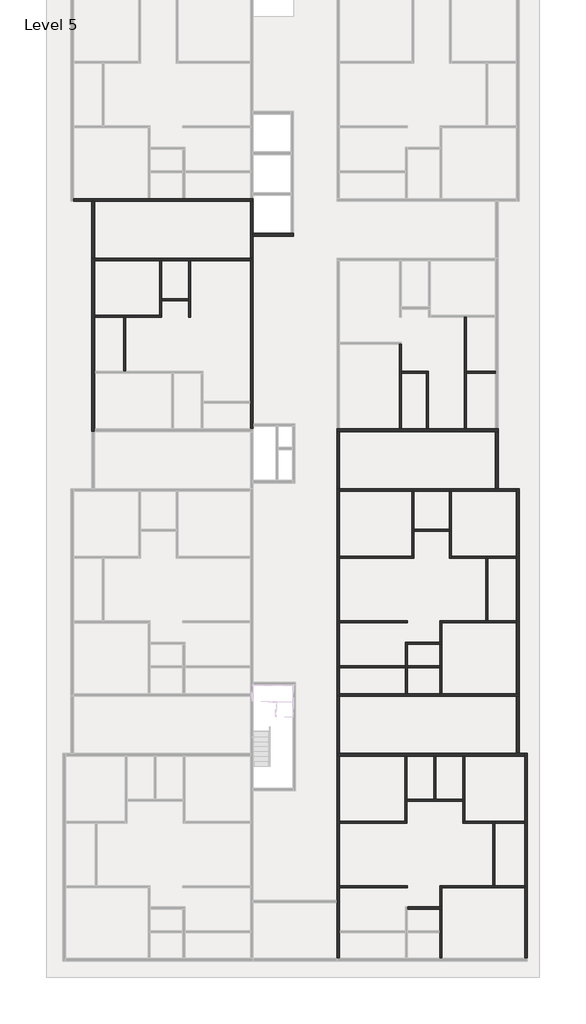
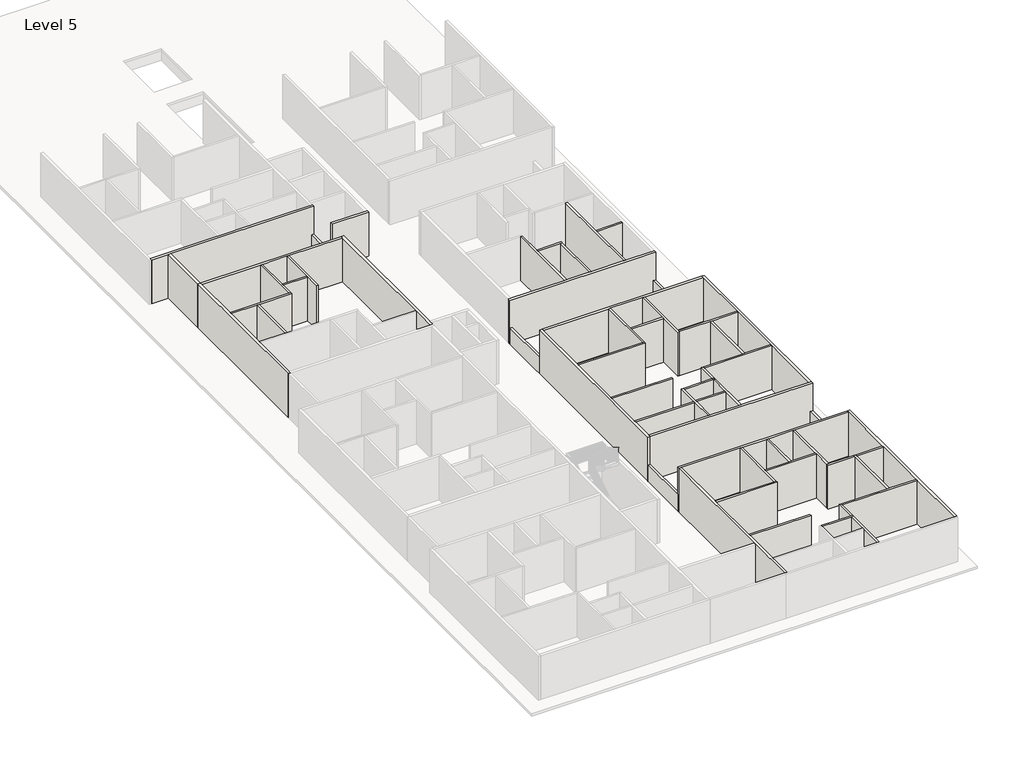
# One storey, part 2 of 8: 56 walls.
"""IFC4 building model written with IfcOpenShell, lengths in millimetres."""

from ifc_helpers import new_model, si_unit, frame, origin, place, context, project, spatial, polyline, outline, extrude, faceted_brep, element, save

model = new_model("IFC4")

# Units and contexts
model_context = context("Model", 3, world=origin())
ifc_project = project(units=[si_unit("LENGTHUNIT", "METRE", prefix="MILLI")], contexts=[model_context])

# Site, building, storey
site = spatial("IfcSite", under=ifc_project)
building = spatial("IfcBuilding", under=site)
storey = spatial("IfcBuildingStorey", under=building, Name="Level 5", Elevation=37426.6172466)

# Walls
placement = place(None, origin())
element("IfcWall", 1, ObjectType="4.5\"", at=placement, inside=storey, context=model_context, shape_type="Brep", body=[
    faceted_brep([(-12531.5544854, 2100.0216096, 37426.6172466), (-10907.2415084, 2100.0216096, 37426.6172466), (-10792.9415084, 2100.0216096, 37426.6172466), (-8759.6544854, 2100.0216096, 37426.6172466), (-8759.6544854, 2100.0216096, 40474.6172466), (-10792.9415084, 2100.0216096, 40474.6172466), (-10907.2415084, 2100.0216096, 40474.6172466), (-12531.5544854, 2100.0216096, 40474.6172466), (-12531.5544854, 2214.3216096, 37426.6172466), (-12531.5544854, 2214.3216096, 40474.6172466), (-8873.9544854, 2214.3216096, 40474.6172466), (-8759.6544854, 2214.3216096, 40474.6172466), (-8759.6544854, 2214.3216096, 37426.6172466), (-8873.9544854, 2214.3216096, 37426.6172466)], [[[0, 1, 2, 3, 4, 5, 6, 7]], [[8, 9, 10, 11, 12, 13]], [[3, 2, 1, 0, 8, 13, 12]], [[0, 7, 9, 8]], [[4, 3, 12, 11]], [[7, 6, 5, 4, 11, 10, 9]]]),
])
element("IfcWall", 2, ObjectType="4.5\"", at=placement, inside=storey, context=model_context, shape_type="Brep", body=[
    faceted_brep([(-8759.6544854, 2214.3216096, 37426.6172466), (-8759.6544854, 3014.4216096, 37426.6172466), (-8759.6544854, 3128.7216096, 37426.6172466), (-8759.6544854, 5264.2743917, 37426.6172466), (-8759.6544854, 5264.2743917, 40474.6172466), (-8759.6544854, 3128.7216096, 40474.6172466), (-8759.6544854, 3014.4216096, 40474.6172466), (-8759.6544854, 2214.3216096, 40474.6172466), (-8873.9544854, 2214.3216096, 37426.6172466), (-8873.9544854, 2214.3216096, 40474.6172466), (-8873.9544854, 5264.2743917, 40474.6172466), (-8873.9544854, 5264.2743917, 37426.6172466)], [[[0, 1, 2, 3, 4, 5, 6, 7]], [[8, 9, 10, 11]], [[3, 2, 1, 0, 8, 11]], [[0, 7, 9, 8]], [[4, 3, 11, 10]], [[7, 6, 5, 4, 10, 9]]]),
])
element("IfcWall", 3, ObjectType="4.5\"", at=placement, inside=storey, context=model_context, shape_type="Brep", body=[
    faceted_brep([(-7235.6544854, 5264.2743917, 37426.6172466), (-7235.6544854, 3128.7216096, 37426.6172466), (-7235.6544854, 3014.4216096, 37426.6172466), (-7235.6544854, 2100.0216096, 37426.6172466), (-7235.6544854, 2100.0216096, 40474.6172466), (-7235.6544854, 3014.4216096, 40474.6172466), (-7235.6544854, 3128.7216096, 40474.6172466), (-7235.6544854, 5264.2743917, 40474.6172466), (-7121.3544854, 5264.2743917, 37426.6172466), (-7121.3544854, 5264.2743917, 40474.6172466), (-7121.3544854, 2100.0216096, 40474.6172466), (-7121.3544854, 2100.0216096, 37426.6172466)], [[[0, 1, 2, 3, 4, 5, 6, 7]], [[8, 9, 10, 11]], [[3, 2, 1, 0, 8, 11]], [[4, 3, 11, 10]], [[0, 7, 9, 8]], [[7, 6, 5, 4, 10, 9]]]),
])
element("IfcWall", 4, ObjectType="4.5\"", at=placement, inside=storey, context=model_context, shape_type="SweptSolid", body=[
    extrude(outline(polyline([(-7235.6544854, 3014.4216096), (-8759.6544854, 3014.4216096), (-8759.6544854, 3128.7216096), (-7235.6544854, 3128.7216096), (-7235.6544854, 3014.4216096)])), frame((0.0, 0.0, 37426.6172466), z_axis=(0.0, 0.0, 1.0), x_axis=(1.0, 0.0, 0.0)), (0.0, 0.0, 1.0), 3048.0),
])
element("IfcWall", 5, ObjectType="4.5\"", at=placement, inside=storey, context=model_context, shape_type="SweptSolid", body=[
    extrude(outline(polyline([(-10907.2415084, -947.4344126), (-10907.2415084, 2100.0216096), (-10792.9415084, 2100.0216096), (-10792.9415084, -947.4344126), (-10907.2415084, -947.4344126)])), frame((0.0, 0.0, 37426.6172466), z_axis=(0.0, 0.0, 1.0), x_axis=(1.0, 0.0, 0.0)), (0.0, 0.0, 1.0), 3048.0),
])
element("IfcWall", 6, ObjectType="4.5\"", at=placement, inside=storey, context=model_context, shape_type="Brep", body=[
    faceted_brep([(5056.6584916, -31173.4344126, 37426.6172466), (6885.4584916, -31173.4344126, 37426.6172466), (6999.7584916, -31173.4344126, 37426.6172466), (6999.7584916, -31173.4344126, 40474.6172466), (6885.4584916, -31173.4344126, 40474.6172466), (5056.6584916, -31173.4344126, 40474.6172466), (5056.6584916, -31059.1344126, 37426.6172466), (5056.6584916, -31059.1344126, 40474.6172466), (6885.4584916, -31059.1344126, 40474.6172466), (6999.7584916, -31059.1344126, 40474.6172466), (6999.7584916, -31059.1344126, 37426.6172466), (6885.4584916, -31059.1344126, 37426.6172466)], [[[0, 1, 2, 3, 4, 5]], [[6, 7, 8, 9, 10, 11]], [[2, 1, 0, 6, 11, 10]], [[0, 5, 7, 6]], [[3, 2, 10, 9]], [[5, 4, 3, 9, 8, 7]]]),
])
element("IfcWall", 7, ObjectType="4.5\"", at=placement, inside=storey, context=model_context, shape_type="Brep", body=[
    faceted_brep([(6885.4584916, -31173.4344126, 37426.6172466), (6885.4584916, -32392.6344126, 37426.6172466), (6885.4584916, -32506.9344126, 37426.6172466), (6885.4584916, -33954.7344126, 37426.6172466), (6885.4584916, -33954.7344126, 40474.6172466), (6885.4584916, -32506.9344126, 40474.6172466), (6885.4584916, -32392.6344126, 40474.6172466), (6885.4584916, -31173.4344126, 40474.6172466), (6999.7584916, -31173.4344126, 37426.6172466), (6999.7584916, -31173.4344126, 40474.6172466), (6999.7584916, -33954.7344126, 40474.6172466), (6999.7584916, -33954.7344126, 37426.6172466)], [[[0, 1, 2, 3, 4, 5, 6, 7]], [[8, 9, 10, 11]], [[3, 2, 1, 0, 8, 11]], [[0, 7, 9, 8]], [[4, 3, 11, 10]], [[7, 6, 5, 4, 10, 9]]]),
])
element("IfcWall", 8, ObjectType="4.5\"", at=placement, inside=storey, context=model_context, shape_type="Brep", body=[
    faceted_brep([(6999.7584916, -31059.1344126, 37426.6172466), (6999.7584916, -29966.9344126, 37426.6172466), (6999.7584916, -29852.6344126, 37426.6172466), (6999.7584916, -29852.6344126, 40474.6172466), (6999.7584916, -29966.9344126, 40474.6172466), (6999.7584916, -31059.1344126, 40474.6172466), (6885.4584916, -31059.1344126, 37426.6172466), (6885.4584916, -31059.1344126, 40474.6172466), (6885.4584916, -29852.6344126, 40474.6172466), (6885.4584916, -29852.6344126, 37426.6172466)], [[[0, 1, 2, 3, 4, 5]], [[6, 7, 8, 9]], [[2, 1, 0, 6, 9]], [[0, 5, 7, 6]], [[3, 2, 9, 8]], [[5, 4, 3, 8, 7]]]),
])
element("IfcWall", 9, ObjectType="4.5\"", at=placement, inside=storey, context=model_context, shape_type="Brep", body=[
    faceted_brep([(6999.7584916, -29966.9344126, 37426.6172466), (11660.6584916, -29966.9344126, 37426.6172466), (11660.6584916, -29966.9344126, 40474.6172466), (6999.7584916, -29966.9344126, 40474.6172466), (6999.7584916, -29852.6344126, 37426.6172466), (6999.7584916, -29852.6344126, 40474.6172466), (9869.9584916, -29852.6344126, 40474.6172466), (9984.2584916, -29852.6344126, 40474.6172466), (11660.6584916, -29852.6344126, 40474.6172466), (11660.6584916, -29852.6344126, 37426.6172466), (9984.2584916, -29852.6344126, 37426.6172466), (9869.9584916, -29852.6344126, 37426.6172466)], [[[0, 1, 2, 3]], [[4, 5, 6, 7, 8, 9, 10, 11]], [[1, 0, 4, 11, 10, 9]], [[0, 3, 5, 4]], [[2, 1, 9, 8]], [[3, 2, 8, 7, 6, 5]]]),
])
element("IfcWall", 10, ObjectType="4.5\"", at=placement, inside=storey, context=model_context, shape_type="SweptSolid", body=[
    extrude(outline(polyline([(5056.6584916, -29966.9344126), (1259.3584916, -29966.9344126), (1259.3584916, -29852.6344126), (5056.6584916, -29852.6344126), (5056.6584916, -29966.9344126)])), frame((0.0, 0.0, 37426.6172466), z_axis=(0.0, 0.0, 1.0), x_axis=(1.0, 0.0, 0.0)), (0.0, 0.0, 1.0), 3048.0),
])
element("IfcWall", 11, ObjectType="4.5\"", at=placement, inside=storey, context=model_context, shape_type="Brep", body=[
    faceted_brep([(1259.3584916, -26347.4344126, 37426.6172466), (5031.2584916, -26347.4344126, 37426.6172466), (5031.2584916, -26347.4344126, 40474.6172466), (1259.3584916, -26347.4344126, 40474.6172466), (1259.3584916, -26233.1344126, 37426.6172466), (1259.3584916, -26233.1344126, 40474.6172466), (4916.9584916, -26233.1344126, 40474.6172466), (5031.2584916, -26233.1344126, 40474.6172466), (5031.2584916, -26233.1344126, 37426.6172466), (4916.9584916, -26233.1344126, 37426.6172466)], [[[0, 1, 2, 3]], [[4, 5, 6, 7, 8, 9]], [[1, 0, 4, 9, 8]], [[0, 3, 5, 4]], [[2, 1, 8, 7]], [[3, 2, 7, 6, 5]]]),
])
element("IfcWall", 12, ObjectType="4.5\"", at=placement, inside=storey, context=model_context, shape_type="Brep", body=[
    faceted_brep([(5031.2584916, -26233.1344126, 37426.6172466), (5031.2584916, -25128.2344126, 37426.6172466), (5031.2584916, -25013.9344126, 37426.6172466), (5031.2584916, -22575.5344126, 37426.6172466), (5031.2584916, -22575.5344126, 40474.6172466), (5031.2584916, -25013.9344126, 40474.6172466), (5031.2584916, -25128.2344126, 40474.6172466), (5031.2584916, -26233.1344126, 40474.6172466), (4916.9584916, -26233.1344126, 37426.6172466), (4916.9584916, -26233.1344126, 40474.6172466), (4916.9584916, -22575.5344126, 40474.6172466), (4916.9584916, -22575.5344126, 37426.6172466)], [[[0, 1, 2, 3, 4, 5, 6, 7]], [[8, 9, 10, 11]], [[3, 2, 1, 0, 8, 11]], [[0, 7, 9, 8]], [[4, 3, 11, 10]], [[7, 6, 5, 4, 10, 9]]]),
])
element("IfcWall", 13, ObjectType="4.5\"", at=placement, inside=storey, context=model_context, shape_type="Brep", body=[
    faceted_brep([(9984.2584916, -29852.6344126, 37426.6172466), (9984.2584916, -26347.4344126, 37426.6172466), (9984.2584916, -26233.1344126, 37426.6172466), (9984.2584916, -26233.1344126, 40474.6172466), (9984.2584916, -26347.4344126, 40474.6172466), (9984.2584916, -29852.6344126, 40474.6172466), (9869.9584916, -29852.6344126, 37426.6172466), (9869.9584916, -29852.6344126, 40474.6172466), (9869.9584916, -26347.4344126, 40474.6172466), (9869.9584916, -26233.1344126, 40474.6172466), (9869.9584916, -26233.1344126, 37426.6172466), (9869.9584916, -26347.4344126, 37426.6172466)], [[[0, 1, 2, 3, 4, 5]], [[6, 7, 8, 9, 10, 11]], [[2, 1, 0, 6, 11, 10]], [[0, 5, 7, 6]], [[3, 2, 10, 9]], [[5, 4, 3, 9, 8, 7]]]),
])
element("IfcWall", 14, ObjectType="4.5\"", at=placement, inside=storey, context=model_context, shape_type="SweptSolid", body=[
    extrude(outline(polyline([(11660.6584916, -26347.4344126), (9984.2584916, -26347.4344126), (9984.2584916, -26233.1344126), (11660.6584916, -26233.1344126), (11660.6584916, -26347.4344126)])), frame((0.0, 0.0, 37426.6172466), z_axis=(0.0, 0.0, 1.0), x_axis=(1.0, 0.0, 0.0)), (0.0, 0.0, 1.0), 3048.0),
])
element("IfcWall", 15, ObjectType="4.5\"", at=placement, inside=storey, context=model_context, shape_type="Brep", body=[
    faceted_brep([(9869.9584916, -26233.1344126, 37426.6172466), (8307.8584916, -26233.1344126, 37426.6172466), (8193.5584916, -26233.1344126, 37426.6172466), (8193.5584916, -26233.1344126, 40474.6172466), (8307.8584916, -26233.1344126, 40474.6172466), (9869.9584916, -26233.1344126, 40474.6172466), (9869.9584916, -26347.4344126, 37426.6172466), (9869.9584916, -26347.4344126, 40474.6172466), (8193.5584916, -26347.4344126, 40474.6172466), (8193.5584916, -26347.4344126, 37426.6172466)], [[[0, 1, 2, 3, 4, 5]], [[6, 7, 8, 9]], [[2, 1, 0, 6, 9]], [[0, 5, 7, 6]], [[3, 2, 9, 8]], [[5, 4, 3, 8, 7]]]),
])
element("IfcWall", 16, ObjectType="4.5\"", at=placement, inside=storey, context=model_context, shape_type="Brep", body=[
    faceted_brep([(8307.8584916, -26233.1344126, 37426.6172466), (8307.8584916, -22575.5344126, 37426.6172466), (8307.8584916, -22575.5344126, 40474.6172466), (8307.8584916, -26233.1344126, 40474.6172466), (8193.5584916, -26233.1344126, 37426.6172466), (8193.5584916, -26233.1344126, 40474.6172466), (8193.5584916, -25128.2344126, 40474.6172466), (8193.5584916, -25013.9344126, 40474.6172466), (8193.5584916, -22575.5344126, 40474.6172466), (8193.5584916, -22575.5344126, 37426.6172466), (8193.5584916, -25013.9344126, 37426.6172466), (8193.5584916, -25128.2344126, 37426.6172466)], [[[0, 1, 2, 3]], [[4, 5, 6, 7, 8, 9, 10, 11]], [[1, 0, 4, 11, 10, 9]], [[0, 3, 5, 4]], [[2, 1, 9, 8]], [[3, 2, 8, 7, 6, 5]]]),
])
element("IfcWall", 17, ObjectType="4.5\"", at=placement, inside=storey, context=model_context, shape_type="Brep", body=[
    faceted_brep([(5031.2584916, -25128.2344126, 37426.6172466), (8193.5584916, -25128.2344126, 37426.6172466), (8193.5584916, -25128.2344126, 40474.6172466), (5031.2584916, -25128.2344126, 40474.6172466), (5031.2584916, -25013.9344126, 37426.6172466), (5031.2584916, -25013.9344126, 40474.6172466), (6555.2584916, -25013.9344126, 40474.6172466), (6669.5584916, -25013.9344126, 40474.6172466), (8193.5584916, -25013.9344126, 40474.6172466), (8193.5584916, -25013.9344126, 37426.6172466), (6669.5584916, -25013.9344126, 37426.6172466), (6555.2584916, -25013.9344126, 37426.6172466)], [[[0, 1, 2, 3]], [[4, 5, 6, 7, 8, 9, 10, 11]], [[1, 0, 4, 11, 10, 9]], [[0, 3, 5, 4]], [[2, 1, 9, 8]], [[3, 2, 8, 7, 6, 5]]]),
])
element("IfcWall", 18, ObjectType="4.5\"", at=placement, inside=storey, context=model_context, shape_type="SweptSolid", body=[
    extrude(outline(polyline([(6555.2584916, -25013.9344126), (6555.2584916, -22575.5344126), (6669.5584916, -22575.5344126), (6669.5584916, -25013.9344126), (6555.2584916, -25013.9344126)])), frame((0.0, 0.0, 37426.6172466), z_axis=(0.0, 0.0, 1.0), x_axis=(1.0, 0.0, 0.0)), (0.0, 0.0, 1.0), 3048.0),
])
element("IfcWall", 19, ObjectType="4.5\"", at=placement, inside=storey, context=model_context, shape_type="SweptSolid", body=[
    extrude(outline(polyline([(4942.3584916, -17622.5344126), (1259.3584916, -17622.5344126), (1259.3584916, -17508.2344126), (4942.3584916, -17508.2344126), (4942.3584916, -17622.5344126)])), frame((0.0, 0.0, 37426.6172466), z_axis=(0.0, 0.0, 1.0), x_axis=(1.0, 0.0, 0.0)), (0.0, 0.0, 1.0), 3048.0),
])
element("IfcWall", 20, ObjectType="4.5\"", at=placement, inside=storey, context=model_context, shape_type="Brep", body=[
    faceted_brep([(4942.3584916, -16174.7344126, 37426.6172466), (4942.3584916, -17508.2344126, 37426.6172466), (4942.3584916, -17622.5344126, 37426.6172466), (4942.3584916, -19070.3344126, 37426.6172466), (4942.3584916, -19070.3344126, 40474.6172466), (4942.3584916, -17622.5344126, 40474.6172466), (4942.3584916, -17508.2344126, 40474.6172466), (4942.3584916, -16174.7344126, 40474.6172466), (5056.6584916, -16174.7344126, 37426.6172466), (5056.6584916, -16174.7344126, 40474.6172466), (5056.6584916, -16289.0344126, 40474.6172466), (5056.6584916, -17508.2344126, 40474.6172466), (5056.6584916, -17622.5344126, 40474.6172466), (5056.6584916, -19070.3344126, 40474.6172466), (5056.6584916, -19070.3344126, 37426.6172466), (5056.6584916, -17622.5344126, 37426.6172466), (5056.6584916, -17508.2344126, 37426.6172466), (5056.6584916, -16289.0344126, 37426.6172466)], [[[0, 1, 2, 3, 4, 5, 6, 7]], [[8, 9, 10, 11, 12, 13, 14, 15, 16, 17]], [[3, 2, 1, 0, 8, 17, 16, 15, 14]], [[4, 3, 14, 13]], [[0, 7, 9, 8]], [[7, 6, 5, 4, 13, 12, 11, 10, 9]]]),
])
element("IfcWall", 21, ObjectType="4.5\"", at=placement, inside=storey, context=model_context, shape_type="Brep", body=[
    faceted_brep([(5056.6584916, -16289.0344126, 37426.6172466), (6885.4584916, -16289.0344126, 37426.6172466), (6999.7584916, -16289.0344126, 37426.6172466), (6999.7584916, -16289.0344126, 40474.6172466), (6885.4584916, -16289.0344126, 40474.6172466), (5056.6584916, -16289.0344126, 40474.6172466), (5056.6584916, -16174.7344126, 37426.6172466), (5056.6584916, -16174.7344126, 40474.6172466), (6885.4584916, -16174.7344126, 40474.6172466), (6999.7584916, -16174.7344126, 40474.6172466), (6999.7584916, -16174.7344126, 37426.6172466), (6885.4584916, -16174.7344126, 37426.6172466)], [[[0, 1, 2, 3, 4, 5]], [[6, 7, 8, 9, 10, 11]], [[2, 1, 0, 6, 11, 10]], [[0, 5, 7, 6]], [[3, 2, 10, 9]], [[5, 4, 3, 9, 8, 7]]]),
])
element("IfcWall", 22, ObjectType="4.5\"", at=placement, inside=storey, context=model_context, shape_type="Brep", body=[
    faceted_brep([(6885.4584916, -16289.0344126, 37426.6172466), (6885.4584916, -17508.2344126, 37426.6172466), (6885.4584916, -17622.5344126, 37426.6172466), (6885.4584916, -19070.3344126, 37426.6172466), (6885.4584916, -19070.3344126, 40474.6172466), (6885.4584916, -17622.5344126, 40474.6172466), (6885.4584916, -17508.2344126, 40474.6172466), (6885.4584916, -16289.0344126, 40474.6172466), (6999.7584916, -16289.0344126, 37426.6172466), (6999.7584916, -16289.0344126, 40474.6172466), (6999.7584916, -19070.3344126, 40474.6172466), (6999.7584916, -19070.3344126, 37426.6172466)], [[[0, 1, 2, 3, 4, 5, 6, 7]], [[8, 9, 10, 11]], [[3, 2, 1, 0, 8, 11]], [[0, 7, 9, 8]], [[4, 3, 11, 10]], [[7, 6, 5, 4, 10, 9]]]),
])
element("IfcWall", 23, ObjectType="4.5\"", at=placement, inside=storey, context=model_context, shape_type="SweptSolid", body=[
    extrude(outline(polyline([(6885.4584916, -17622.5344126), (5056.6584916, -17622.5344126), (5056.6584916, -17508.2344126), (6885.4584916, -17508.2344126), (6885.4584916, -17622.5344126)])), frame((0.0, 0.0, 37426.6172466), z_axis=(0.0, 0.0, 1.0), x_axis=(1.0, 0.0, 0.0)), (0.0, 0.0, 1.0), 3048.0),
])
element("IfcWall", 24, ObjectType="4.5\"", at=placement, inside=storey, context=model_context, shape_type="Brep", body=[
    faceted_brep([(6999.7584916, -16174.7344126, 37426.6172466), (6999.7584916, -15082.5344126, 37426.6172466), (6999.7584916, -14968.2344126, 37426.6172466), (6999.7584916, -14968.2344126, 40474.6172466), (6999.7584916, -15082.5344126, 40474.6172466), (6999.7584916, -16174.7344126, 40474.6172466), (6885.4584916, -16174.7344126, 37426.6172466), (6885.4584916, -16174.7344126, 40474.6172466), (6885.4584916, -14968.2344126, 40474.6172466), (6885.4584916, -14968.2344126, 37426.6172466)], [[[0, 1, 2, 3, 4, 5]], [[6, 7, 8, 9]], [[2, 1, 0, 6, 9]], [[0, 5, 7, 6]], [[3, 2, 9, 8]], [[5, 4, 3, 8, 7]]]),
])
element("IfcWall", 25, ObjectType="4.5\"", at=placement, inside=storey, context=model_context, shape_type="Brep", body=[
    faceted_brep([(6999.7584916, -15082.5344126, 37426.6172466), (11208.5214687, -15082.5344126, 37426.6172466), (11208.5214687, -15082.5344126, 40474.6172466), (6999.7584916, -15082.5344126, 40474.6172466), (6999.7584916, -14968.2344126, 37426.6172466), (6999.7584916, -14968.2344126, 40474.6172466), (9469.9084916, -14968.2344126, 40474.6172466), (9584.2084916, -14968.2344126, 40474.6172466), (11208.5214687, -14968.2344126, 40474.6172466), (11208.5214687, -14968.2344126, 37426.6172466), (9584.2084916, -14968.2344126, 37426.6172466), (9469.9084916, -14968.2344126, 37426.6172466)], [[[0, 1, 2, 3]], [[4, 5, 6, 7, 8, 9, 10, 11]], [[1, 0, 4, 11, 10, 9]], [[0, 3, 5, 4]], [[2, 1, 9, 8]], [[3, 2, 8, 7, 6, 5]]]),
])
element("IfcWall", 26, ObjectType="4.5\"", at=placement, inside=storey, context=model_context, shape_type="SweptSolid", body=[
    extrude(outline(polyline([(5056.6584916, -15082.5344126), (1259.3584916, -15082.5344126), (1259.3584916, -14968.2344126), (5056.6584916, -14968.2344126), (5056.6584916, -15082.5344126)])), frame((0.0, 0.0, 37426.6172466), z_axis=(0.0, 0.0, 1.0), x_axis=(1.0, 0.0, 0.0)), (0.0, 0.0, 1.0), 3048.0),
])
element("IfcWall", 27, ObjectType="4.5\"", at=placement, inside=storey, context=model_context, shape_type="Brep", body=[
    faceted_brep([(1259.3584916, -11463.0344126, 37426.6172466), (5430.0214687, -11463.0344126, 37426.6172466), (5430.0214687, -11463.0344126, 40474.6172466), (1259.3584916, -11463.0344126, 40474.6172466), (1259.3584916, -11348.7344126, 37426.6172466), (1259.3584916, -11348.7344126, 40474.6172466), (5315.7214687, -11348.7344126, 40474.6172466), (5430.0214687, -11348.7344126, 40474.6172466), (5430.0214687, -11348.7344126, 37426.6172466), (5315.7214687, -11348.7344126, 37426.6172466)], [[[0, 1, 2, 3]], [[4, 5, 6, 7, 8, 9]], [[1, 0, 4, 9, 8]], [[0, 3, 5, 4]], [[2, 1, 8, 7]], [[3, 2, 7, 6, 5]]]),
])
element("IfcWall", 28, ObjectType="4.5\"", at=placement, inside=storey, context=model_context, shape_type="Brep", body=[
    faceted_brep([(5430.0214687, -11348.7344126, 37426.6172466), (5430.0214687, -9939.0344126, 37426.6172466), (5430.0214687, -9824.7344126, 37426.6172466), (5430.0214687, -7691.1344126, 37426.6172466), (5430.0214687, -7691.1344126, 40474.6172466), (5430.0214687, -9824.7344126, 40474.6172466), (5430.0214687, -9939.0344126, 40474.6172466), (5430.0214687, -11348.7344126, 40474.6172466), (5315.7214687, -11348.7344126, 37426.6172466), (5315.7214687, -11348.7344126, 40474.6172466), (5315.7214687, -7691.1344126, 40474.6172466), (5315.7214687, -7691.1344126, 37426.6172466)], [[[0, 1, 2, 3, 4, 5, 6, 7]], [[8, 9, 10, 11]], [[3, 2, 1, 0, 8, 11]], [[0, 7, 9, 8]], [[4, 3, 11, 10]], [[7, 6, 5, 4, 10, 9]]]),
])
element("IfcWall", 29, ObjectType="4.5\"", at=placement, inside=storey, context=model_context, shape_type="SweptSolid", body=[
    extrude(outline(polyline([(7436.6214687, -9939.0344126), (5430.0214687, -9939.0344126), (5430.0214687, -9824.7344126), (7436.6214687, -9824.7344126), (7436.6214687, -9939.0344126)])), frame((0.0, 0.0, 37426.6172466), z_axis=(0.0, 0.0, 1.0), x_axis=(1.0, 0.0, 0.0)), (0.0, 0.0, 1.0), 3048.0),
])
element("IfcWall", 30, ObjectType="4.5\"", at=placement, inside=storey, context=model_context, shape_type="Brep", body=[
    faceted_brep([(7436.6214687, -7691.1344126, 37426.6172466), (7436.6214687, -9824.7344126, 37426.6172466), (7436.6214687, -9939.0344126, 37426.6172466), (7436.6214687, -11463.0344126, 37426.6172466), (7436.6214687, -11463.0344126, 40474.6172466), (7436.6214687, -9939.0344126, 40474.6172466), (7436.6214687, -9824.7344126, 40474.6172466), (7436.6214687, -7691.1344126, 40474.6172466), (7550.9214687, -7691.1344126, 37426.6172466), (7550.9214687, -7691.1344126, 40474.6172466), (7550.9214687, -11348.7344126, 40474.6172466), (7550.9214687, -11463.0344126, 40474.6172466), (7550.9214687, -11463.0344126, 37426.6172466), (7550.9214687, -11348.7344126, 37426.6172466)], [[[0, 1, 2, 3, 4, 5, 6, 7]], [[8, 9, 10, 11, 12, 13]], [[3, 2, 1, 0, 8, 13, 12]], [[0, 7, 9, 8]], [[4, 3, 12, 11]], [[7, 6, 5, 4, 11, 10, 9]]]),
])
element("IfcWall", 31, ObjectType="4.5\"", at=placement, inside=storey, context=model_context, shape_type="Brep", body=[
    faceted_brep([(7550.9214687, -11463.0344126, 37426.6172466), (9469.9084916, -11463.0344126, 37426.6172466), (9584.2084916, -11463.0344126, 37426.6172466), (11208.5214687, -11463.0344126, 37426.6172466), (11208.5214687, -11463.0344126, 40474.6172466), (9584.2084916, -11463.0344126, 40474.6172466), (9469.9084916, -11463.0344126, 40474.6172466), (7550.9214687, -11463.0344126, 40474.6172466), (7550.9214687, -11348.7344126, 37426.6172466), (7550.9214687, -11348.7344126, 40474.6172466), (11208.5214687, -11348.7344126, 40474.6172466), (11208.5214687, -11348.7344126, 37426.6172466)], [[[0, 1, 2, 3, 4, 5, 6, 7]], [[8, 9, 10, 11]], [[3, 2, 1, 0, 8, 11]], [[0, 7, 9, 8]], [[4, 3, 11, 10]], [[7, 6, 5, 4, 10, 9]]]),
])
element("IfcWall", 32, ObjectType="4.5\"", at=placement, inside=storey, context=model_context, shape_type="SweptSolid", body=[
    extrude(outline(polyline([(9469.9084916, -14968.2344126), (9469.9084916, -11463.0344126), (9584.2084916, -11463.0344126), (9584.2084916, -14968.2344126), (9469.9084916, -14968.2344126)])), frame((0.0, 0.0, 37426.6172466), z_axis=(0.0, 0.0, 1.0), x_axis=(1.0, 0.0, 0.0)), (0.0, 0.0, 1.0), 3048.0),
])
element("IfcWall", 33, ObjectType="4.5\"", at=placement, inside=storey, context=model_context, shape_type="Brep", body=[
    faceted_brep([(4610.8714687, 572.7745083, 37426.6172466), (4610.8714687, -4185.9344126, 37426.6172466), (4610.8714687, -4185.9344126, 40474.6172466), (4610.8714687, 572.7745083, 40474.6172466), (4725.1714687, 572.7745083, 37426.6172466), (4725.1714687, 572.7745083, 40474.6172466), (4725.1714687, -947.4344126, 40474.6172466), (4725.1714687, -1061.7344126, 40474.6172466), (4725.1714687, -4185.9344126, 40474.6172466), (4725.1714687, -4185.9344126, 37426.6172466), (4725.1714687, -1061.7344126, 37426.6172466), (4725.1714687, -947.4344126, 37426.6172466)], [[[0, 1, 2, 3]], [[4, 5, 6, 7, 8, 9, 10, 11]], [[1, 0, 4, 11, 10, 9]], [[0, 3, 5, 4]], [[2, 1, 9, 8]], [[3, 2, 8, 7, 6, 5]]]),
])
element("IfcWall", 34, ObjectType="4.5\"", at=placement, inside=storey, context=model_context, shape_type="Brep", body=[
    faceted_brep([(4725.1714687, -1061.7344126, 37426.6172466), (6134.8714687, -1061.7344126, 37426.6172466), (6249.1714687, -1061.7344126, 37426.6172466), (6249.1714687, -1061.7344126, 40474.6172466), (6134.8714687, -1061.7344126, 40474.6172466), (4725.1714687, -1061.7344126, 40474.6172466), (4725.1714687, -947.4344126, 37426.6172466), (4725.1714687, -947.4344126, 40474.6172466), (6249.1714687, -947.4344126, 40474.6172466), (6249.1714687, -947.4344126, 37426.6172466)], [[[0, 1, 2, 3, 4, 5]], [[6, 7, 8, 9]], [[2, 1, 0, 6, 9]], [[0, 5, 7, 6]], [[3, 2, 9, 8]], [[5, 4, 3, 8, 7]]]),
])
element("IfcWall", 35, ObjectType="4.5\"", at=placement, inside=storey, context=model_context, shape_type="SweptSolid", body=[
    extrude(outline(polyline([(6134.8714687, -4185.9344126), (6134.8714687, -1061.7344126), (6249.1714687, -1061.7344126), (6249.1714687, -4185.9344126), (6134.8714687, -4185.9344126)])), frame((0.0, 0.0, 37426.6172466), z_axis=(0.0, 0.0, 1.0), x_axis=(1.0, 0.0, 0.0)), (0.0, 0.0, 1.0), 3048.0),
])
element("IfcWall", 36, ObjectType="4.5\"", at=placement, inside=storey, context=model_context, shape_type="Brep", body=[
    faceted_brep([(8396.7584916, -4185.9344126, 37426.6172466), (8396.7584916, -1061.7344126, 37426.6172466), (8396.7584916, -947.4344126, 37426.6172466), (8396.7584916, 2100.0216096, 37426.6172466), (8396.7584916, 2100.0216096, 40474.6172466), (8396.7584916, -947.4344126, 40474.6172466), (8396.7584916, -1061.7344126, 40474.6172466), (8396.7584916, -4185.9344126, 40474.6172466), (8282.4584916, -4185.9344126, 37426.6172466), (8282.4584916, -4185.9344126, 40474.6172466), (8282.4584916, 2100.0216096, 40474.6172466), (8282.4584916, 2100.0216096, 37426.6172466)], [[[0, 1, 2, 3, 4, 5, 6, 7]], [[8, 9, 10, 11]], [[3, 2, 1, 0, 8, 11]], [[0, 7, 9, 8]], [[4, 3, 11, 10]], [[7, 6, 5, 4, 10, 9]]]),
])
element("IfcWall", 37, ObjectType="4.5\"", at=placement, inside=storey, context=model_context, shape_type="SweptSolid", body=[
    extrude(outline(polyline([(8396.7584916, -947.4344126), (10021.0714687, -947.4344126), (10021.0714687, -1061.7344126), (8396.7584916, -1061.7344126), (8396.7584916, -947.4344126)])), frame((0.0, 0.0, 37426.6172466), z_axis=(0.0, 0.0, 1.0), x_axis=(1.0, 0.0, 0.0)), (0.0, 0.0, 1.0), 3048.0),
])
element("IfcWall", 38, ObjectType="6\"", at=placement, inside=storey, context=model_context, shape_type="Brep", body=[
    faceted_brep([(-13719.0044854, 8615.1216096, 37426.6172466), (-12683.9544854, 8615.1216096, 37426.6172466), (-12531.5544854, 8615.1216096, 37426.6172466), (-3769.8415084, 8615.1216096, 37426.6172466), (-3617.4415084, 8615.1216096, 37426.6172466), (-3617.4415084, 8615.1216096, 38645.8172466), (-3617.4415084, 8615.1216096, 40474.6172466), (-12531.5544854, 8615.1216096, 40474.6172466), (-12683.9544854, 8615.1216096, 40474.6172466), (-13719.0044854, 8615.1216096, 40474.6172466), (-13719.0044854, 8767.5216096, 37426.6172466), (-13719.0044854, 8767.5216096, 40474.6172466), (-9510.2415084, 8767.5216096, 40474.6172466), (-9395.9415084, 8767.5216096, 40474.6172466), (-7567.1415084, 8767.5216096, 40474.6172466), (-7452.8415084, 8767.5216096, 40474.6172466), (-3769.8415084, 8767.5216096, 40474.6172466), (-3617.4415084, 8767.5216096, 40474.6172466), (-3617.4415084, 8767.5216096, 37426.6172466), (-3769.8415084, 8767.5216096, 37426.6172466), (-7452.8415084, 8767.5216096, 37426.6172466), (-7567.1415084, 8767.5216096, 37426.6172466), (-9395.9415084, 8767.5216096, 37426.6172466), (-9510.2415084, 8767.5216096, 37426.6172466)], [[[0, 1, 2, 3, 4, 5, 6, 7, 8, 9]], [[10, 11, 12, 13, 14, 15, 16, 17, 18, 19, 20, 21, 22, 23]], [[4, 3, 2, 1, 0, 10, 23, 22, 21, 20, 19, 18]], [[0, 9, 11, 10]], [[4, 18, 17, 6, 5]], [[9, 8, 7, 6, 17, 16, 15, 14, 13, 12, 11]]]),
])
element("IfcWall", 39, ObjectType="6\"", at=placement, inside=storey, context=model_context, shape_type="Brep", body=[
    faceted_brep([(-12683.9544854, 5416.6743917, 37426.6172466), (-12683.9544854, -4338.3344126, 37426.6172466), (-12683.9544854, -4338.3344126, 40474.6172466), (-12683.9544854, 5416.6743917, 40474.6172466), (-12531.5544854, 5416.6743917, 37426.6172466), (-12531.5544854, 5416.6743917, 40474.6172466), (-12531.5544854, 5264.2743917, 40474.6172466), (-12531.5544854, 2214.3216096, 40474.6172466), (-12531.5544854, 2100.0216096, 40474.6172466), (-12531.5544854, -947.4344126, 40474.6172466), (-12531.5544854, -1061.7344126, 40474.6172466), (-12531.5544854, -4185.9344126, 40474.6172466), (-12531.5544854, -4338.3344126, 40474.6172466), (-12531.5544854, -4338.3344126, 37426.6172466), (-12531.5544854, -4185.9344126, 37426.6172466), (-12531.5544854, -1061.7344126, 37426.6172466), (-12531.5544854, -947.4344126, 37426.6172466), (-12531.5544854, 2100.0216096, 37426.6172466), (-12531.5544854, 2214.3216096, 37426.6172466), (-12531.5544854, 5264.2743917, 37426.6172466)], [[[0, 1, 2, 3]], [[4, 5, 6, 7, 8, 9, 10, 11, 12, 13, 14, 15, 16, 17, 18, 19]], [[1, 0, 4, 19, 18, 17, 16, 15, 14, 13]], [[2, 1, 13, 12]], [[0, 3, 5, 4]], [[3, 2, 12, 11, 10, 9, 8, 7, 6, 5]]]),
])
element("IfcWall", 40, ObjectType="6\"", at=placement, inside=storey, context=model_context, shape_type="Brep", body=[
    faceted_brep([(-3617.4415084, -4185.9344126, 37426.6172466), (-3617.4415084, -4034.6751812, 37426.6172466), (-3617.4415084, -3882.2751812, 37426.6172466), (-3617.4415084, 5416.6743917, 37426.6172466), (-3617.4415084, 5416.6743917, 40474.6172466), (-3617.4415084, -3882.2751812, 40474.6172466), (-3617.4415084, -4034.6751812, 40474.6172466), (-3617.4415084, -4185.9344126, 40474.6172466), (-3769.8415084, -4185.9344126, 37426.6172466), (-3769.8415084, -4185.9344126, 40474.6172466), (-3769.8415084, -2738.1344126, 40474.6172466), (-3769.8415084, -2623.8344126, 40474.6172466), (-3769.8415084, 5264.2743917, 40474.6172466), (-3769.8415084, 5416.6743917, 40474.6172466), (-3769.8415084, 5416.6743917, 37426.6172466), (-3769.8415084, 5264.2743917, 37426.6172466), (-3769.8415084, -2623.8344126, 37426.6172466), (-3769.8415084, -2738.1344126, 37426.6172466)], [[[0, 1, 2, 3, 4, 5, 6, 7]], [[8, 9, 10, 11, 12, 13, 14, 15, 16, 17]], [[3, 2, 1, 0, 8, 17, 16, 15, 14]], [[0, 7, 9, 8]], [[3, 14, 13, 4]], [[7, 6, 5, 4, 13, 12, 11, 10, 9]]]),
])
element("IfcWall", 41, ObjectType="6\"", at=placement, inside=storey, context=model_context, shape_type="Brep", body=[
    faceted_brep([(-3769.8415084, 5416.6743917, 40474.6172466), (-3769.8415084, 5416.6743917, 37426.6172466), (-12531.5544854, 5416.6743917, 37426.6172466), (-12531.5544854, 5416.6743917, 40474.6172466), (-3769.8415084, 5264.2743917, 37426.6172466), (-3769.8415084, 5264.2743917, 40474.6172466), (-7121.3544854, 5264.2743917, 40474.6172466), (-7235.6544854, 5264.2743917, 40474.6172466), (-8759.6544854, 5264.2743917, 40474.6172466), (-8873.9544854, 5264.2743917, 40474.6172466), (-12531.5544854, 5264.2743917, 40474.6172466), (-12531.5544854, 5264.2743917, 37426.6172466), (-8873.9544854, 5264.2743917, 37426.6172466), (-8759.6544854, 5264.2743917, 37426.6172466), (-7235.6544854, 5264.2743917, 37426.6172466), (-7121.3544854, 5264.2743917, 37426.6172466)], [[[0, 1, 2, 3]], [[4, 5, 6, 7, 8, 9, 10, 11, 12, 13, 14, 15]], [[2, 1, 4, 15, 14, 13, 12, 11]], [[3, 2, 11, 10]], [[0, 5, 4, 1]], [[0, 3, 10, 9, 8, 7, 6, 5]]]),
])
element("IfcWall", 42, ObjectType="6\"", at=placement, inside=storey, context=model_context, shape_type="Brep", body=[
    faceted_brep([(11813.0584916, -33954.7344126, 37426.6172466), (11813.0584916, -22423.1344126, 37426.6172466), (11813.0584916, -22423.1344126, 40474.6172466), (11813.0584916, -33954.7344126, 40474.6172466), (11660.6584916, -33954.7344126, 37426.6172466), (11660.6584916, -33954.7344126, 40474.6172466), (11660.6584916, -29966.9344126, 40474.6172466), (11660.6584916, -29852.6344126, 40474.6172466), (11660.6584916, -26347.4344126, 40474.6172466), (11660.6584916, -26233.1344126, 40474.6172466), (11660.6584916, -22575.5344126, 40474.6172466), (11660.6584916, -22423.1344126, 40474.6172466), (11660.6584916, -22423.1344126, 37426.6172466), (11660.6584916, -22575.5344126, 37426.6172466), (11660.6584916, -26233.1344126, 37426.6172466), (11660.6584916, -26347.4344126, 37426.6172466), (11660.6584916, -29852.6344126, 37426.6172466), (11660.6584916, -29966.9344126, 37426.6172466)], [[[0, 1, 2, 3]], [[4, 5, 6, 7, 8, 9, 10, 11, 12, 13, 14, 15, 16, 17]], [[1, 0, 4, 17, 16, 15, 14, 13, 12]], [[0, 3, 5, 4]], [[2, 1, 12, 11]], [[3, 2, 11, 10, 9, 8, 7, 6, 5]]]),
])
element("IfcWall", 43, ObjectType="6\"", at=placement, inside=storey, context=model_context, shape_type="Brep", body=[
    faceted_brep([(11660.6584916, -22423.1344126, 37426.6172466), (11360.9214687, -22423.1344126, 37426.6172466), (11208.5214687, -22423.1344126, 37426.6172466), (1259.3584916, -22423.1344126, 37426.6172466), (1106.9584916, -22423.1344126, 37426.6172466), (1106.9584916, -22423.1344126, 38645.8172466), (1106.9584916, -22423.1344126, 40474.6172466), (11660.6584916, -22423.1344126, 40474.6172466), (11660.6584916, -22575.5344126, 37426.6172466), (11660.6584916, -22575.5344126, 40474.6172466), (8307.8584916, -22575.5344126, 40474.6172466), (8193.5584916, -22575.5344126, 40474.6172466), (6669.5584916, -22575.5344126, 40474.6172466), (6555.2584916, -22575.5344126, 40474.6172466), (5031.2584916, -22575.5344126, 40474.6172466), (4916.9584916, -22575.5344126, 40474.6172466), (1259.3584916, -22575.5344126, 40474.6172466), (1106.9584916, -22575.5344126, 40474.6172466), (1106.9584916, -22575.5344126, 37426.6172466), (1259.3584916, -22575.5344126, 37426.6172466), (4916.9584916, -22575.5344126, 37426.6172466), (5031.2584916, -22575.5344126, 37426.6172466), (6555.2584916, -22575.5344126, 37426.6172466), (6669.5584916, -22575.5344126, 37426.6172466), (8193.5584916, -22575.5344126, 37426.6172466), (8307.8584916, -22575.5344126, 37426.6172466)], [[[0, 1, 2, 3, 4, 5, 6, 7]], [[8, 9, 10, 11, 12, 13, 14, 15, 16, 17, 18, 19, 20, 21, 22, 23, 24, 25]], [[4, 3, 2, 1, 0, 8, 25, 24, 23, 22, 21, 20, 19, 18]], [[0, 7, 9, 8]], [[4, 18, 17, 6, 5]], [[7, 6, 17, 16, 15, 14, 13, 12, 11, 10, 9]]]),
])
element("IfcWall", 44, ObjectType="6\"", at=placement, inside=storey, context=model_context, shape_type="Brep", body=[
    faceted_brep([(1106.9584916, -22575.5344126, 40474.6172466), (1106.9584916, -22575.5344126, 37426.6172466), (1106.9584916, -30668.5325185, 37426.6172466), (1106.9584916, -30820.9325185, 37426.6172466), (1106.9584916, -33954.7344126, 37426.6172466), (1106.9584916, -33954.7344126, 40474.6172466), (1106.9584916, -30820.9325185, 40474.6172466), (1106.9584916, -30668.5325185, 40474.6172466), (1259.3584916, -22575.5344126, 37426.6172466), (1259.3584916, -22575.5344126, 40474.6172466), (1259.3584916, -26233.1344126, 40474.6172466), (1259.3584916, -26347.4344126, 40474.6172466), (1259.3584916, -29852.6344126, 40474.6172466), (1259.3584916, -29966.9344126, 40474.6172466), (1259.3584916, -32392.6344126, 40474.6172466), (1259.3584916, -32506.9344126, 40474.6172466), (1259.3584916, -33954.7344126, 40474.6172466), (1259.3584916, -33954.7344126, 37426.6172466), (1259.3584916, -32506.9344126, 37426.6172466), (1259.3584916, -32392.6344126, 37426.6172466), (1259.3584916, -29966.9344126, 37426.6172466), (1259.3584916, -29852.6344126, 37426.6172466), (1259.3584916, -26347.4344126, 37426.6172466), (1259.3584916, -26233.1344126, 37426.6172466)], [[[0, 1, 2, 3, 4, 5, 6, 7]], [[8, 9, 10, 11, 12, 13, 14, 15, 16, 17, 18, 19, 20, 21, 22, 23]], [[4, 3, 2, 1, 8, 23, 22, 21, 20, 19, 18, 17]], [[5, 4, 17, 16]], [[0, 9, 8, 1]], [[0, 7, 6, 5, 16, 15, 14, 13, 12, 11, 10, 9]]]),
])
element("IfcWall", 45, ObjectType="6\"", at=placement, inside=storey, context=model_context, shape_type="Brep", body=[
    faceted_brep([(1106.9584916, -7538.7344126, 40474.6172466), (1106.9584916, -7538.7344126, 37426.6172466), (1106.9584916, -19222.7344126, 37426.6172466), (1106.9584916, -19222.7344126, 40474.6172466), (1259.3584916, -7538.7344126, 37426.6172466), (1259.3584916, -7538.7344126, 40474.6172466), (1259.3584916, -7691.1344126, 40474.6172466), (1259.3584916, -11348.7344126, 40474.6172466), (1259.3584916, -11463.0344126, 40474.6172466), (1259.3584916, -14968.2344126, 40474.6172466), (1259.3584916, -15082.5344126, 40474.6172466), (1259.3584916, -17508.2344126, 40474.6172466), (1259.3584916, -17622.5344126, 40474.6172466), (1259.3584916, -19070.3344126, 40474.6172466), (1259.3584916, -19222.7344126, 40474.6172466), (1259.3584916, -19222.7344126, 37426.6172466), (1259.3584916, -19070.3344126, 37426.6172466), (1259.3584916, -17622.5344126, 37426.6172466), (1259.3584916, -17508.2344126, 37426.6172466), (1259.3584916, -15082.5344126, 37426.6172466), (1259.3584916, -14968.2344126, 37426.6172466), (1259.3584916, -11463.0344126, 37426.6172466), (1259.3584916, -11348.7344126, 37426.6172466), (1259.3584916, -7691.1344126, 37426.6172466)], [[[0, 1, 2, 3]], [[4, 5, 6, 7, 8, 9, 10, 11, 12, 13, 14, 15, 16, 17, 18, 19, 20, 21, 22, 23]], [[2, 1, 4, 23, 22, 21, 20, 19, 18, 17, 16, 15]], [[0, 5, 4, 1]], [[2, 15, 14, 3]], [[0, 3, 14, 13, 12, 11, 10, 9, 8, 7, 6, 5]]]),
])
element("IfcWall", 46, ObjectType="6\"", at=placement, inside=storey, context=model_context, shape_type="Brep", body=[
    faceted_brep([(1259.3584916, -19222.7344126, 40474.6172466), (1259.3584916, -19222.7344126, 37426.6172466), (11208.5214687, -19222.7344126, 37426.6172466), (11360.9214687, -19222.7344126, 37426.6172466), (11360.9214687, -19222.7344126, 38645.8172466), (11360.9214687, -19222.7344126, 40474.6172466), (1259.3584916, -19070.3344126, 37426.6172466), (1259.3584916, -19070.3344126, 40474.6172466), (4942.3584916, -19070.3344126, 40474.6172466), (5056.6584916, -19070.3344126, 40474.6172466), (6885.4584916, -19070.3344126, 40474.6172466), (6999.7584916, -19070.3344126, 40474.6172466), (11208.5214687, -19070.3344126, 40474.6172466), (11360.9214687, -19070.3344126, 40474.6172466), (11360.9214687, -19070.3344126, 37426.6172466), (11208.5214687, -19070.3344126, 37426.6172466), (6999.7584916, -19070.3344126, 37426.6172466), (6885.4584916, -19070.3344126, 37426.6172466), (5056.6584916, -19070.3344126, 37426.6172466), (4942.3584916, -19070.3344126, 37426.6172466)], [[[0, 1, 2, 3, 4, 5]], [[6, 7, 8, 9, 10, 11, 12, 13, 14, 15, 16, 17, 18, 19]], [[3, 2, 1, 6, 19, 18, 17, 16, 15, 14]], [[3, 14, 13, 5, 4]], [[0, 7, 6, 1]], [[0, 5, 13, 12, 11, 10, 9, 8, 7]]]),
])
element("IfcWall", 47, ObjectType="6\"", at=placement, inside=storey, context=model_context, shape_type="Brep", body=[
    faceted_brep([(11360.9214687, -19070.3344126, 40474.6172466), (11360.9214687, -19070.3344126, 37426.6172466), (11360.9214687, -7538.7344126, 37426.6172466), (11360.9214687, -7538.7344126, 40474.6172466), (11208.5214687, -19070.3344126, 37426.6172466), (11208.5214687, -19070.3344126, 40474.6172466), (11208.5214687, -15082.5344126, 40474.6172466), (11208.5214687, -14968.2344126, 40474.6172466), (11208.5214687, -11463.0344126, 40474.6172466), (11208.5214687, -11348.7344126, 40474.6172466), (11208.5214687, -7691.1344126, 40474.6172466), (11208.5214687, -7538.7344126, 40474.6172466), (11208.5214687, -7538.7344126, 37426.6172466), (11208.5214687, -7691.1344126, 37426.6172466), (11208.5214687, -11348.7344126, 37426.6172466), (11208.5214687, -11463.0344126, 37426.6172466), (11208.5214687, -14968.2344126, 37426.6172466), (11208.5214687, -15082.5344126, 37426.6172466)], [[[0, 1, 2, 3]], [[4, 5, 6, 7, 8, 9, 10, 11, 12, 13, 14, 15, 16, 17]], [[2, 1, 4, 17, 16, 15, 14, 13, 12]], [[3, 2, 12, 11]], [[0, 5, 4, 1]], [[0, 3, 11, 10, 9, 8, 7, 6, 5]]]),
])
element("IfcWall", 48, ObjectType="6\"", at=placement, inside=storey, context=model_context, shape_type="Brep", body=[
    faceted_brep([(11208.5214687, -7538.7344126, 37426.6172466), (10173.4714687, -7538.7344126, 37426.6172466), (10021.0714687, -7538.7344126, 37426.6172466), (1259.3584916, -7538.7344126, 37426.6172466), (1259.3584916, -7538.7344126, 40474.6172466), (11208.5214687, -7538.7344126, 40474.6172466), (11208.5214687, -7691.1344126, 37426.6172466), (11208.5214687, -7691.1344126, 40474.6172466), (7550.9214687, -7691.1344126, 40474.6172466), (7436.6214687, -7691.1344126, 40474.6172466), (5430.0214687, -7691.1344126, 40474.6172466), (5315.7214687, -7691.1344126, 40474.6172466), (1259.3584916, -7691.1344126, 40474.6172466), (1259.3584916, -7691.1344126, 37426.6172466), (5315.7214687, -7691.1344126, 37426.6172466), (5430.0214687, -7691.1344126, 37426.6172466), (7436.6214687, -7691.1344126, 37426.6172466), (7550.9214687, -7691.1344126, 37426.6172466)], [[[0, 1, 2, 3, 4, 5]], [[6, 7, 8, 9, 10, 11, 12, 13, 14, 15, 16, 17]], [[3, 2, 1, 0, 6, 17, 16, 15, 14, 13]], [[0, 5, 7, 6]], [[3, 13, 12, 4]], [[5, 4, 12, 11, 10, 9, 8, 7]]]),
])
element("IfcWall", 49, ObjectType="6\"", at=placement, inside=storey, context=model_context, shape_type="Brep", body=[
    faceted_brep([(1106.9584916, -4338.3344126, 40474.6172466), (1106.9584916, -4338.3344126, 38645.8172466), (1106.9584916, -4338.3344126, 37426.6172466), (1259.3584916, -4338.3344126, 37426.6172466), (10021.0714687, -4338.3344126, 37426.6172466), (10173.4714687, -4338.3344126, 37426.6172466), (10173.4714687, -4338.3344126, 38645.8172466), (10173.4714687, -4338.3344126, 40474.6172466), (1106.9584916, -4185.9344126, 37426.6172466), (1106.9584916, -4185.9344126, 40474.6172466), (1259.3584916, -4185.9344126, 40474.6172466), (4610.8714687, -4185.9344126, 40474.6172466), (4725.1714687, -4185.9344126, 40474.6172466), (6134.8714687, -4185.9344126, 40474.6172466), (6249.1714687, -4185.9344126, 40474.6172466), (8282.4584916, -4185.9344126, 40474.6172466), (8396.7584916, -4185.9344126, 40474.6172466), (10021.0714687, -4185.9344126, 40474.6172466), (10173.4714687, -4185.9344126, 40474.6172466), (10173.4714687, -4185.9344126, 37426.6172466), (10021.0714687, -4185.9344126, 37426.6172466), (8396.7584916, -4185.9344126, 37426.6172466), (8282.4584916, -4185.9344126, 37426.6172466), (6249.1714687, -4185.9344126, 37426.6172466), (6134.8714687, -4185.9344126, 37426.6172466), (4725.1714687, -4185.9344126, 37426.6172466), (4610.8714687, -4185.9344126, 37426.6172466), (1259.3584916, -4185.9344126, 37426.6172466)], [[[0, 1, 2, 3, 4, 5, 6, 7]], [[8, 9, 10, 11, 12, 13, 14, 15, 16, 17, 18, 19, 20, 21, 22, 23, 24, 25, 26, 27]], [[5, 4, 3, 2, 8, 27, 26, 25, 24, 23, 22, 21, 20, 19]], [[0, 9, 8, 2, 1]], [[5, 19, 18, 7, 6]], [[0, 7, 18, 17, 16, 15, 14, 13, 12, 11, 10, 9]]]),
])
element("IfcWall", 50, ObjectType="6\"", at=placement, inside=storey, context=model_context, shape_type="Brep", body=[
    faceted_brep([(-3617.4415084, 6659.2303368, 37426.6172466), (-1331.4415084, 6659.2303368, 37426.6172466), (-1331.4415084, 6659.2303368, 40474.6172466), (-3617.4415084, 6659.2303368, 40474.6172466), (-3617.4415084, 6811.6303368, 37426.6172466), (-3617.4415084, 6811.6303368, 40474.6172466), (-1483.8415084, 6811.6303368, 40474.6172466), (-1331.4415084, 6811.6303368, 40474.6172466), (-1331.4415084, 6811.6303368, 37426.6172466), (-1483.8415084, 6811.6303368, 37426.6172466)], [[[0, 1, 2, 3]], [[4, 5, 6, 7, 8, 9]], [[1, 0, 4, 9, 8]], [[3, 2, 7, 6, 5]], [[0, 3, 5, 4]], [[2, 1, 8, 7]]]),
])
element("IfcWall", 51, ObjectType="6\" 2", at=placement, inside=storey, context=model_context, shape_type="SweptSolid", body=[
    extrude(outline(polyline([(-12683.9544854, 5416.6743917), (-12683.9544854, 8615.1216096), (-12531.5544854, 8615.1216096), (-12531.5544854, 5416.6743917), (-12683.9544854, 5416.6743917)])), frame((0.0, 0.0, 37426.6172466), z_axis=(0.0, 0.0, 1.0), x_axis=(1.0, 0.0, 0.0)), (0.0, 0.0, 1.0), 3048.0),
])
element("IfcWall", 52, ObjectType="6\" 2", at=placement, inside=storey, context=model_context, shape_type="Brep", body=[
    faceted_brep([(-3769.8415084, 8615.1216096, 37426.6172466), (-3769.8415084, 5416.6743917, 37426.6172466), (-3769.8415084, 5416.6743917, 38645.8172466), (-3769.8415084, 8615.1216096, 38645.8172466), (-3617.4415084, 8615.1216096, 37426.6172466), (-3617.4415084, 8615.1216096, 38645.8172466), (-3617.4415084, 5416.6743917, 38645.8172466), (-3617.4415084, 5416.6743917, 37426.6172466), (-3617.4415084, 6659.2303368, 37426.6172466), (-3617.4415084, 6811.6303368, 37426.6172466)], [[[0, 1, 2, 3]], [[4, 5, 6, 7, 8, 9]], [[1, 0, 4, 9, 8, 7]], [[3, 2, 6, 5]], [[0, 3, 5, 4]], [[2, 1, 7, 6]]]),
])
element("IfcWall", 53, ObjectType="6\" 2", at=placement, inside=storey, context=model_context, shape_type="SweptSolid", body=[
    extrude(outline(polyline([(1106.9584916, -7538.7344126), (1106.9584916, -4338.3344126), (1259.3584916, -4338.3344126), (1259.3584916, -7538.7344126), (1106.9584916, -7538.7344126)])), frame((0.0, 0.0, 37426.6172466), z_axis=(0.0, 0.0, 1.0), x_axis=(1.0, 0.0, 0.0)), (0.0, 0.0, 1.0), 1219.2),
])
element("IfcWall", 54, ObjectType="6\" 2", at=placement, inside=storey, context=model_context, shape_type="SweptSolid", body=[
    extrude(outline(polyline([(10021.0714687, -7538.7344126), (10021.0714687, -4338.3344126), (10173.4714687, -4338.3344126), (10173.4714687, -7538.7344126), (10021.0714687, -7538.7344126)])), frame((0.0, 0.0, 37426.6172466), z_axis=(0.0, 0.0, 1.0), x_axis=(1.0, 0.0, 0.0)), (0.0, 0.0, 1.0), 1219.2),
])
element("IfcWall", 55, ObjectType="6\" 2", at=placement, inside=storey, context=model_context, shape_type="SweptSolid", body=[
    extrude(outline(polyline([(11208.5214687, -22423.1344126), (11208.5214687, -19222.7344126), (11360.9214687, -19222.7344126), (11360.9214687, -22423.1344126), (11208.5214687, -22423.1344126)])), frame((0.0, 0.0, 37426.6172466), z_axis=(0.0, 0.0, 1.0), x_axis=(1.0, 0.0, 0.0)), (0.0, 0.0, 1.0), 1219.2),
])
element("IfcWall", 56, ObjectType="6\" 2", at=placement, inside=storey, context=model_context, shape_type="SweptSolid", body=[
    extrude(outline(polyline([(1106.9584916, -22423.1344126), (1106.9584916, -19222.7344126), (1259.3584916, -19222.7344126), (1259.3584916, -22423.1344126), (1106.9584916, -22423.1344126)])), frame((0.0, 0.0, 37426.6172466), z_axis=(0.0, 0.0, 1.0), x_axis=(1.0, 0.0, 0.0)), (0.0, 0.0, 1.0), 1219.2),
])

save(model, "model.ifc")

# Revit data of these elements
# Type "4.5\""
#   Assembly Code = "B2010"
#   Layers, outside or top first: 0' - 4 1/2" "WALLS" (function 1)
# Type "6\""
#   Assembly Code = "B2010"
#   Layers, outside or top first: 0' - 6" "WALLS" (function 1)
# Type "6\" 2"
#   Assembly Code = "B2010"
#   Layers, outside or top first: 0' - 6" "4'" (function 1)
# Elements 1, 2, 3, 4, 5, 6, 7, 8, 9, 10, 11, 12, 13, 14, 15, 16, 17, 18, 19, 20, 21, 22, 23, 24, 25, 26, 27, 28, 29, 30, 31, 32, 33, 34, 35, 36, 37 (IfcWall, "4.5\"")
#   Top Offset = 0' - 0"
#   Base Offset = 0' - 0"
#   Unconnected Height = 10' - 0"
#   wall height = 10' - 0"
#   Phase Created = New Construction
#   Base Constraint = Level 5
#   Materials on its faces: "WALLS"
# Elements 38, 39, 40, 41, 42, 43, 44, 45, 46, 47, 48, 49, 50 (IfcWall, "6\"")
#   Top Offset = 0' - 0"
#   Base Offset = 0' - 0"
#   Unconnected Height = 10' - 0"
#   wall height = 10' - 0"
#   Phase Created = New Construction
#   Base Constraint = Level 5
#   Materials on its faces: "WALLS"
# Element 51 (IfcWall, "6\" 2")
#   Top Offset = 0' - 0"
#   Base Offset = 0' - 0"
#   Unconnected Height = 10' - 0"
#   wall height = 10' - 0"
#   Phase Created = New Construction
#   Base Constraint = Level 5
#   Materials on its faces: "4'"
# Elements 52, 53, 54, 55, 56 (IfcWall, "6\" 2")
#   Top Offset = 0' - 0"
#   Base Offset = 0' - 0"
#   Unconnected Height = 4' - 0"
#   wall height = 4' - 0"
#   Phase Created = New Construction
#   Base Constraint = Level 5
#   Materials on its faces: "4'"
# Materials
#   "WALLS": class "Generic", colour RGB 120 120 120, transparency 0, Cost = 0
#   "4'": class "Generic", colour RGB 120 120 120, transparency 0, Cost = 0
